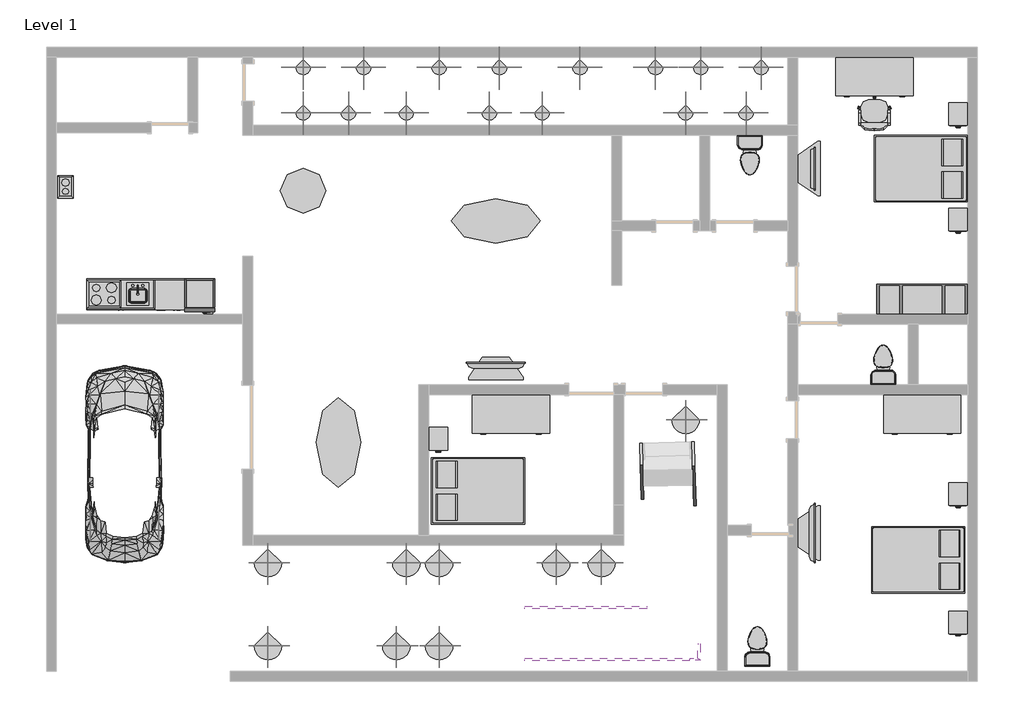
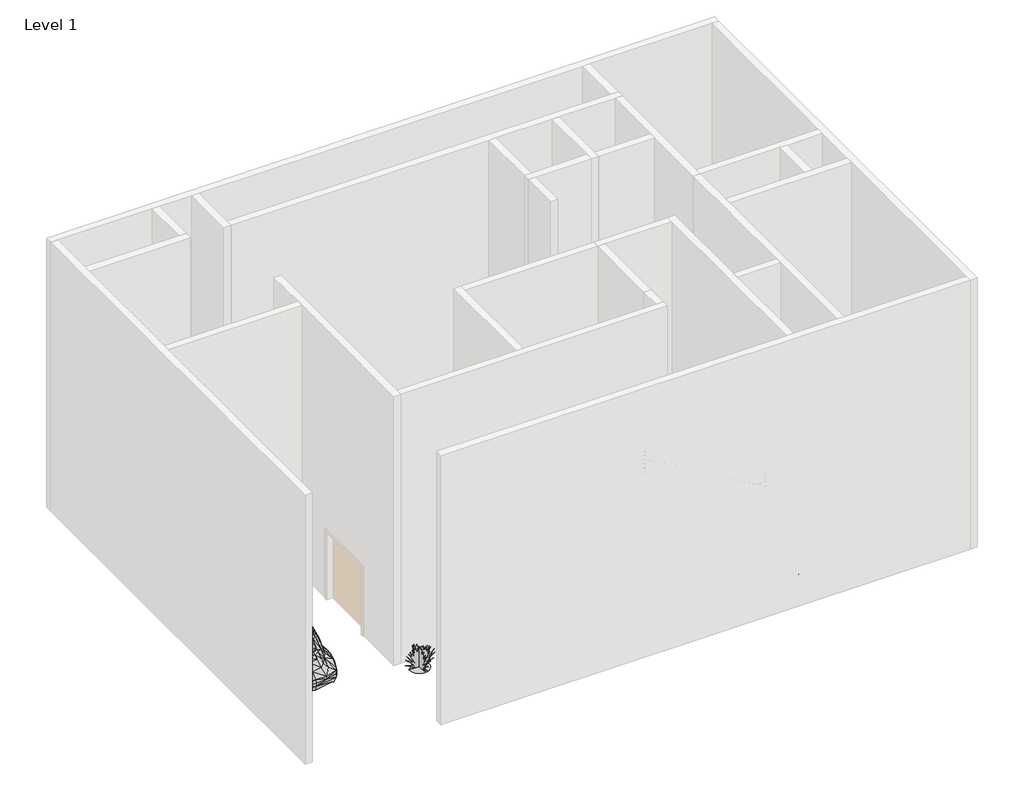
# One storey, part 4 of 4: 24 geographic elements, 23 furniture elements, 6 members, 6 proxies, 4 flow terminals.
"""IFC4 building model written with IfcOpenShell, lengths in millimetres."""

from ifc_helpers import new_model, si_unit, frame, origin, place, context, project, spatial, polyline, outline, extrude, faceted_brep, transform, mapped, element, save
from components import m_cook_top_2_unit_305_x_457mm_ebea1746, m_cook_top_4_unit2_0615_x_500mm_249f3515, m_dishwasher_610_x_610_x_875mm_54ecfc4c, m_kitchenette_medium_1372mm_e05c6bec, m_rpc_beetle_m_rpc_beetle_b6d71803, m_refrigerator_600_x_660mm_a466bf94, m_sink_kitchen_island_450_x_450mm_f969cf2d, m_toilet_domestic_3d_m_toilet_domestic_3d_5cb52bd4, m_toilet_domestic_3d_m_toilet_domestic_3d_183bbd19, m_toilet_domestic_3d_m_toilet_domestic_3d_43425dfb, m_toilet_domestic_3d_m_toilet_domestic_3d_5530cc89, furniture_40ec15d9, furniture_0810mm_56245f3a, furniture_1190mm_d9bcc661, m_bed_box_1346_x_1880mm_double_b32eb57e, m_cabinet_file_2_drawer_0380_x_0457mm_9eec7cff, m_chair_executive_m_chair_executive_8d69e98c, m_counter_top_w_sink_hole_600mm_depth_0a237b63, m_desk_1525_x_762mm_8f660baf, m_entertainment_center_1830_x_1830_x_0610mm_f77a9b93, m_table_dining_round_w_chairs_0915mm_diameter_5defa876, m_table_ellipse_1800_x_900mm_fd46d5a5, m_rpc_plant_tropical_agave_0_45_meters_eb57889b, m_rpc_plant_tropical_dagger_0_6_meters_5dc34e47

model = new_model("IFC4")

# Units and contexts
model_context = context("Model", 3, world=origin())
ifc_project = project(units=[si_unit("LENGTHUNIT", "METRE", prefix="MILLI")], contexts=[model_context])

# Site, building, storey
site = spatial("IfcSite", under=ifc_project)
building = spatial("IfcBuilding", under=site)
storey = spatial("IfcBuildingStorey", under=building, Name="Level 1", Elevation=0.0)

# Proxies
placement = place(None, origin())
m_cook_top_2_unit_305_x_457mm_shape = m_cook_top_2_unit_305_x_457mm_ebea1746(model_context)
element("IfcBuildingElementProxy", 1, Name="M_Cook Top-2 Unit : 305 x 457mm", ObjectType="M_Cook Top-2 Unit : 305 x 457mm", at=placement, inside=storey, context=model_context, shape_type="MappedRepresentation", body=[
    mapped(m_cook_top_2_unit_305_x_457mm_shape, transform((-9406.4268643, 7109.0723156, 0.0), x_axis=(1.0, 0.0, 0.0), y_axis=(0.0, 1.0, 0.0), z_axis=(0.0, 0.0, 1.0))),
])
m_cook_top_4_unit2_0615_x_500mm_shape = m_cook_top_4_unit2_0615_x_500mm_249f3515(model_context)
element("IfcBuildingElementProxy", 2, Name="M_Cook Top-4 Unit2 : 0615 x 500mm", ObjectType="M_Cook Top-4 Unit2 : 0615 x 500mm", at=placement, inside=storey, context=model_context, shape_type="MappedRepresentation", body=[
    mapped(m_cook_top_4_unit2_0615_x_500mm_shape, transform((-8555.8268643, 4978.8971112, 0.0), x_axis=(1.0, 0.0, 0.0), y_axis=(0.0, 1.0, 0.0), z_axis=(0.0, 0.0, 1.0))),
])
m_dishwasher_610_x_610_x_875mm_shape = m_dishwasher_610_x_610_x_875mm_54ecfc4c(model_context)
element("IfcBuildingElementProxy", 3, Name="M_Dishwasher : 610 x 610 x 875mm", ObjectType="M_Dishwasher : 610 x 610 x 875mm", at=placement, inside=storey, context=model_context, shape_type="MappedRepresentation", body=[
    mapped(m_dishwasher_610_x_610_x_875mm_shape, transform((-7606.3443328, 4712.2475464, 0.0), x_axis=(1.0, 0.0, 0.0), y_axis=(0.0, 1.0, 0.0), z_axis=(0.0, 0.0, 1.0))),
])
m_kitchenette_medium_1372mm_shape = m_kitchenette_medium_1372mm_e05c6bec(model_context)
element("IfcBuildingElementProxy", 4, Name="M_Kitchenette - Medium : 1372mm", ObjectType="M_Kitchenette - Medium : 1372mm", at=placement, inside=storey, context=model_context, shape_type="MappedRepresentation", body=[
    mapped(m_kitchenette_medium_1372mm_shape, transform((-8231.5645692, 5283.8971112, 0.0), x_axis=(1.0, 0.0, 0.0), y_axis=(0.0, 1.0, 0.0), z_axis=(0.0, 0.0, 1.0))),
])
m_rpc_beetle_m_rpc_beetle_shape = m_rpc_beetle_m_rpc_beetle_b6d71803(model_context)
element("IfcBuildingElementProxy", 5, Name="M_RPC Beetle : M_RPC Beetle", ObjectType="M_RPC Beetle : M_RPC Beetle", at=placement, inside=storey, context=model_context, shape_type="MappedRepresentation", body=[
    mapped(m_rpc_beetle_m_rpc_beetle_shape, transform((-8136.4268643, 306.6971112, 0.0), x_axis=(1.0, 0.0, 0.0), y_axis=(0.0, 1.0, 0.0), z_axis=(0.0, 0.0, 1.0))),
])
m_refrigerator_600_x_660mm_shape = m_refrigerator_600_x_660mm_a466bf94(model_context)
element("IfcBuildingElementProxy", 6, Name="M_Refrigerator : 600 x 660mm", ObjectType="M_Refrigerator : 600 x 660mm", at=placement, inside=storey, context=model_context, shape_type="MappedRepresentation", body=[
    mapped(m_refrigerator_600_x_660mm_shape, transform((-6565.0257216, 4987.682021, 0.0), x_axis=(1.0, 0.0, 0.0), y_axis=(0.0, 1.0, 0.0), z_axis=(0.0, 0.0, 1.0))),
])

# Flow terminals
m_sink_kitchen_island_450_x_450mm_shape = m_sink_kitchen_island_450_x_450mm_f969cf2d(model_context)
element("IfcFlowTerminal", 7, ObjectType="M_Sink Kitchen-Island : 450 x 450mm", at=placement, inside=storey, context=model_context, shape_type="MappedRepresentation", body=[
    mapped(m_sink_kitchen_island_450_x_450mm_shape, transform((-7885.5161048, 4976.5517101, 0.0), x_axis=(1.0, 0.0, 0.0), y_axis=(0.0, 1.0, 0.0), z_axis=(0.0, 0.0, 1.0))),
])
m_toilet_domestic_3d_m_toilet_domestic_3d_shape = m_toilet_domestic_3d_m_toilet_domestic_3d_5cb52bd4(model_context)
m_toilet_domestic_3d_m_toilet_domestic_3d_2_shape = m_toilet_domestic_3d_m_toilet_domestic_3d_183bbd19(model_context)
element("IfcFlowTerminal", 8, ObjectType="M_Toilet-Domestic-3D : M_Toilet-Domestic-3D", at=placement, inside=storey, context=model_context, shape_type="MappedRepresentation", body=[
    mapped(m_toilet_domestic_3d_m_toilet_domestic_3d_shape, transform((4486.3771084, 7686.0010839, 0.0), x_axis=(1.0, 0.0, 0.0), y_axis=(0.0, 1.0, 0.0), z_axis=(0.0, 0.0, 1.0))),
    mapped(m_toilet_domestic_3d_m_toilet_domestic_3d_2_shape, transform((4486.3771084, 7686.0010839, 0.0), x_axis=(1.0, 0.0, 0.0), y_axis=(0.0, 1.0, 0.0), z_axis=(0.0, 0.0, 1.0))),
])
element("IfcFlowTerminal", 9, ObjectType="M_Toilet-Domestic-3D : M_Toilet-Domestic-3D", at=placement, inside=storey, context=model_context, shape_type="MappedRepresentation", body=[
    mapped(m_toilet_domestic_3d_m_toilet_domestic_3d_shape, transform((4637.5691631, -2043.4068614, 0.0), x_axis=(-1.0000000000000004, 0.0, 0.0), y_axis=(0.0, -1.0000000000000004, 0.0), z_axis=(0.0, 0.0, 1.0))),
    mapped(m_toilet_domestic_3d_m_toilet_domestic_3d_2_shape, transform((4637.5691631, -2043.4068614, 0.0), x_axis=(-1.0000000000000004, 0.0, 0.0), y_axis=(0.0, -1.0000000000000004, 0.0), z_axis=(0.0, 0.0, 1.0))),
])
m_toilet_domestic_3d_m_toilet_domestic_3d_3_shape = m_toilet_domestic_3d_m_toilet_domestic_3d_43425dfb(model_context)
m_toilet_domestic_3d_m_toilet_domestic_3d_4_shape = m_toilet_domestic_3d_m_toilet_domestic_3d_5530cc89(model_context)
element("IfcFlowTerminal", 10, ObjectType="M_Toilet-Domestic-3D : M_Toilet-Domestic-3D", at=placement, inside=storey, context=model_context, shape_type="MappedRepresentation", body=[
    mapped(m_toilet_domestic_3d_m_toilet_domestic_3d_3_shape, transform((7177.1771084, 3642.6010839, 0.0), x_axis=(1.0, 0.0, 0.0), y_axis=(0.0, 1.0, 0.0), z_axis=(0.0, 0.0, 1.0))),
    mapped(m_toilet_domestic_3d_m_toilet_domestic_3d_4_shape, transform((7177.1771084, 3642.6010839, 0.0), x_axis=(1.0, 0.0, 0.0), y_axis=(0.0, 1.0, 0.0), z_axis=(0.0, 0.0, 1.0))),
])

# Furniture
furniture_shape = furniture_40ec15d9(model_context)
element("IfcFurniture", 11, at=placement, inside=storey, context=model_context, shape_type="MappedRepresentation", body=[
    mapped(furniture_shape, transform((5449.3731357, 7382.5091092, 0.0), x_axis=(0.0, 1.0000000000000002, 0.0), y_axis=(-1.0000000000000002, 0.0, 0.0), z_axis=(0.0, 0.0, 1.0))),
])
element("IfcFurniture", 12, at=placement, inside=storey, context=model_context, shape_type="MappedRepresentation", body=[
    mapped(furniture_shape, transform((5449.3731357, 25.9091092, 0.0), x_axis=(0.0, 1.0000000000000009, 0.0), y_axis=(-1.0000000000000009, 0.0, 0.0), z_axis=(0.0, 0.0, 1.0))),
])
element("IfcFurniture", 13, at=placement, inside=storey, context=model_context, shape_type="MappedRepresentation", body=[
    mapped(furniture_shape, transform((-768.6148663, 3703.8971112, 0.0), x_axis=(1.0, 0.0, 0.0), y_axis=(0.0, 1.0, 0.0), z_axis=(0.0, 0.0, 1.0))),
])
furniture_0810mm_shape = furniture_0810mm_56245f3a(model_context)
element("IfcFurniture", 14, ObjectType="0810mm", at=placement, inside=storey, context=model_context, shape_type="MappedRepresentation", body=[
    mapped(furniture_0810mm_shape, transform((5737.9117594, 7511.6416254, 0.0), x_axis=(0.0, 1.0, 0.0), y_axis=(-1.0, 0.0, 0.0), z_axis=(0.0, 0.0, 1.0))),
])
furniture_1190mm_shape = furniture_1190mm_d9bcc661(model_context)
element("IfcFurniture", 15, ObjectType="1190mm", at=placement, inside=storey, context=model_context, shape_type="MappedRepresentation", body=[
    mapped(furniture_1190mm_shape, transform((5737.9117594, 155.0416254, 0.0), x_axis=(0.0, 1.0, 0.0), y_axis=(-1.0, 0.0, 0.0), z_axis=(0.0, 0.0, 1.0))),
])
element("IfcFurniture", 16, ObjectType="1190mm", at=placement, inside=storey, context=model_context, shape_type="MappedRepresentation", body=[
    mapped(furniture_1190mm_shape, transform((-647.3713784, 3532.4357349, 0.0), x_axis=(-1.0000000000000002, 0.0, 0.0), y_axis=(0.0, -1.0000000000000002, 0.0), z_axis=(0.0, 0.0, 1.0))),
])
m_bed_box_1346_x_1880mm_double_shape = m_bed_box_1346_x_1880mm_double_b32eb57e(model_context)
element("IfcFurniture", 17, ObjectType="M_Bed-Box : 1346 x 1880mm - Double", at=placement, inside=storey, context=model_context, shape_type="MappedRepresentation", body=[
    mapped(m_bed_box_1346_x_1880mm_double_shape, transform((8174.4026439, 7846.8495702, 0.0), x_axis=(0.0, -1.0000000000000007, 0.0), y_axis=(1.0000000000000007, 0.0, 0.0), z_axis=(0.0, 0.0, 1.0))),
])
element("IfcFurniture", 18, ObjectType="M_Bed-Box : 1346 x 1880mm - Double", at=placement, inside=storey, context=model_context, shape_type="MappedRepresentation", body=[
    mapped(m_bed_box_1346_x_1880mm_double_shape, transform((8119.0026439, -51.1504298, 0.0), x_axis=(0.0, -1.0000000000000004, 0.0), y_axis=(1.0000000000000004, 0.0, 0.0), z_axis=(0.0, 0.0, 1.0))),
])
element("IfcFurniture", 19, ObjectType="M_Bed-Box : 1346 x 1880mm - Double", at=placement, inside=storey, context=model_context, shape_type="MappedRepresentation", body=[
    mapped(m_bed_box_1346_x_1880mm_double_shape, transform((-1238.0563725, 662.9446522, 0.0), x_axis=(0.0, 0.9999999999999999, 0.0), y_axis=(-0.9999999999999999, 0.0, 0.0), z_axis=(0.0, 0.0, 1.0))),
])
m_cabinet_file_2_drawer_0380_x_0457mm_shape = m_cabinet_file_2_drawer_0380_x_0457mm_9eec7cff(model_context)
element("IfcFurniture", 20, ObjectType="M_Cabinet-File 2 Drawer : 0380 x 0457mm", at=placement, inside=storey, context=model_context, shape_type="MappedRepresentation", body=[
    mapped(m_cabinet_file_2_drawer_0380_x_0457mm_shape, transform((8817.8695828, 6622.5314113, 0.0), x_axis=(1.0, 0.0, 0.0), y_axis=(0.0, 1.0, 0.0), z_axis=(0.0, 0.0, 1.0))),
])
element("IfcFurniture", 21, ObjectType="M_Cabinet-File 2 Drawer : 0380 x 0457mm", at=placement, inside=storey, context=model_context, shape_type="MappedRepresentation", body=[
    mapped(m_cabinet_file_2_drawer_0380_x_0457mm_shape, transform((8817.8695828, 8751.3314113, 0.0), x_axis=(1.0, 0.0, 0.0), y_axis=(0.0, 1.0, 0.0), z_axis=(0.0, 0.0, 1.0))),
])
element("IfcFurniture", 22, ObjectType="M_Cabinet-File 2 Drawer : 0380 x 0457mm", at=placement, inside=storey, context=model_context, shape_type="MappedRepresentation", body=[
    mapped(m_cabinet_file_2_drawer_0380_x_0457mm_shape, transform((8817.8695828, 1080.7314113, 0.0), x_axis=(1.0, 0.0, 0.0), y_axis=(0.0, 1.0, 0.0), z_axis=(0.0, 0.0, 1.0))),
])
element("IfcFurniture", 23, ObjectType="M_Cabinet-File 2 Drawer : 0380 x 0457mm", at=placement, inside=storey, context=model_context, shape_type="MappedRepresentation", body=[
    mapped(m_cabinet_file_2_drawer_0380_x_0457mm_shape, transform((8817.8695828, -1510.0685887, 0.0), x_axis=(1.0, 0.0, 0.0), y_axis=(0.0, 1.0, 0.0), z_axis=(0.0, 0.0, 1.0))),
])
element("IfcFurniture", 24, ObjectType="M_Cabinet-File 2 Drawer : 0380 x 0457mm", at=placement, inside=storey, context=model_context, shape_type="MappedRepresentation", body=[
    mapped(m_cabinet_file_2_drawer_0380_x_0457mm_shape, transform((-1676.5304172, 2198.3314113, 0.0), x_axis=(1.0, 0.0, 0.0), y_axis=(0.0, 1.0, 0.0), z_axis=(0.0, 0.0, 1.0))),
])
m_chair_executive_m_chair_executive_shape = m_chair_executive_m_chair_executive_8d69e98c(model_context)
element("IfcFurniture", 25, ObjectType="M_Chair-Executive : M_Chair-Executive", at=placement, inside=storey, context=model_context, shape_type="MappedRepresentation", body=[
    mapped(m_chair_executive_m_chair_executive_shape, transform((6857.2823161, 8620.5512096, 0.0), x_axis=(1.0, 0.0, 0.0), y_axis=(0.0, 1.0, 0.0), z_axis=(0.0, 0.0, 1.0))),
])
m_counter_top_w_sink_hole_600mm_depth_shape = m_counter_top_w_sink_hole_600mm_depth_0a237b63(model_context)
element("IfcFurniture", 26, ObjectType="M_Counter Top w Sink Hole : 600mm Depth", at=placement, inside=storey, context=model_context, shape_type="MappedRepresentation", body=[
    mapped(m_counter_top_w_sink_hole_600mm_depth_shape, transform((-7698.3645692, 5283.8971112, 0.0), x_axis=(1.0, 0.0, 0.0), y_axis=(0.0, 1.0, 0.0), z_axis=(0.0, 0.0, 1.0))),
])
m_desk_1525_x_762mm_shape = m_desk_1525_x_762mm_8f660baf(model_context)
element("IfcFurniture", 27, ObjectType="M_Desk : 1525 x 762mm", at=placement, inside=storey, context=model_context, shape_type="MappedRepresentation", body=[
    mapped(m_desk_1525_x_762mm_shape, transform((6236.2731357, 8996.6971112, 0.0), x_axis=(1.0, 0.0, 0.0), y_axis=(0.0, 1.0, 0.0), z_axis=(0.0, 0.0, 1.0))),
])
element("IfcFurniture", 28, ObjectType="M_Desk : 1525 x 762mm", at=placement, inside=storey, context=model_context, shape_type="MappedRepresentation", body=[
    mapped(m_desk_1525_x_762mm_shape, transform((7202.9731357, 2184.6971112, 0.0), x_axis=(1.0, 0.0, 0.0), y_axis=(0.0, 1.0, 0.0), z_axis=(0.0, 0.0, 1.0))),
])
element("IfcFurniture", 29, ObjectType="M_Desk : 1525 x 762mm", at=placement, inside=storey, context=model_context, shape_type="MappedRepresentation", body=[
    mapped(m_desk_1525_x_762mm_shape, transform((-1101.1268643, 2184.6971112, 0.0), x_axis=(1.0, 0.0, 0.0), y_axis=(0.0, 1.0, 0.0), z_axis=(0.0, 0.0, 1.0))),
])
m_entertainment_center_1830_x_1830_x_0610mm_shape = m_entertainment_center_1830_x_1830_x_0610mm_f77a9b93(model_context)
element("IfcFurniture", 30, ObjectType="M_Entertainment center : 1830 x 1830 x 0610mm", at=placement, inside=storey, context=model_context, shape_type="MappedRepresentation", body=[
    mapped(m_entertainment_center_1830_x_1830_x_0610mm_shape, transform((7964.9731357, 5277.2971112, 0.0), x_axis=(1.0, 0.0, 0.0), y_axis=(0.0, 1.0, 0.0), z_axis=(0.0, 0.0, 1.0))),
])
m_table_dining_round_w_chairs_0915mm_diameter_shape = m_table_dining_round_w_chairs_0915mm_diameter_5defa876(model_context)
element("IfcFurniture", 31, ObjectType="M_Table-Dining Round w Chairs : 0915mm Diameter", at=placement, inside=storey, context=model_context, shape_type="MappedRepresentation", body=[
    mapped(m_table_dining_round_w_chairs_0915mm_diameter_shape, transform((-4636.5088315, 7246.3757997, 0.0), x_axis=(1.0, 0.0, 0.0), y_axis=(0.0, 1.0, 0.0), z_axis=(0.0, 0.0, 1.0))),
])
m_table_ellipse_1800_x_900mm_shape = m_table_ellipse_1800_x_900mm_fd46d5a5(model_context)
element("IfcFurniture", 32, ObjectType="M_Table-Ellipse : 1800 x 900mm", at=placement, inside=storey, context=model_context, shape_type="MappedRepresentation", body=[
    mapped(m_table_ellipse_1800_x_900mm_shape, transform((-643.4268643, 6451.8971112, 0.0), x_axis=(1.0, 0.0, 0.0), y_axis=(0.0, 1.0, 0.0), z_axis=(0.0, 0.0, 1.0))),
])
element("IfcFurniture", 33, ObjectType="M_Table-Ellipse : 1800 x 900mm", at=placement, inside=storey, context=model_context, shape_type="MappedRepresentation", body=[
    mapped(m_table_ellipse_1800_x_900mm_shape, transform((-3821.6268643, 1979.8971112, 0.0), x_axis=(0.0, 1.0000000000000002, 0.0), y_axis=(-1.0000000000000002, 0.0, 0.0), z_axis=(0.0, 0.0, 1.0))),
])

# Geographic elements
m_rpc_plant_tropical_agave_0_45_meters_shape = m_rpc_plant_tropical_agave_0_45_meters_eb57889b(model_context)
element("IfcGeographicElement", 34, ObjectType="M_RPC Plant - Tropical : Agave - 0.45 Meters", at=placement, inside=storey, context=model_context, shape_type="MappedRepresentation", body=[
    mapped(m_rpc_plant_tropical_agave_0_45_meters_shape, transform((-4531.4235354, 9553.8971112, 0.0), x_axis=(1.0, 0.0, 0.0), y_axis=(0.0, 1.0, 0.0), z_axis=(0.0, 0.0, 1.0))),
])
element("IfcGeographicElement", 35, ObjectType="M_RPC Plant - Tropical : Agave - 0.45 Meters", at=placement, inside=storey, context=model_context, shape_type="MappedRepresentation", body=[
    mapped(m_rpc_plant_tropical_agave_0_45_meters_shape, transform((-3312.2235354, 9553.8971112, 0.0), x_axis=(1.0, 0.0, 0.0), y_axis=(0.0, 1.0, 0.0), z_axis=(0.0, 0.0, 1.0))),
])
element("IfcGeographicElement", 36, ObjectType="M_RPC Plant - Tropical : Agave - 0.45 Meters", at=placement, inside=storey, context=model_context, shape_type="MappedRepresentation", body=[
    mapped(m_rpc_plant_tropical_agave_0_45_meters_shape, transform((-1788.2235354, 9553.8971112, 0.0), x_axis=(1.0, 0.0, 0.0), y_axis=(0.0, 1.0, 0.0), z_axis=(0.0, 0.0, 1.0))),
])
element("IfcGeographicElement", 37, ObjectType="M_RPC Plant - Tropical : Agave - 0.45 Meters", at=placement, inside=storey, context=model_context, shape_type="MappedRepresentation", body=[
    mapped(m_rpc_plant_tropical_agave_0_45_meters_shape, transform((-569.0235354, 9553.8971112, 0.0), x_axis=(1.0, 0.0, 0.0), y_axis=(0.0, 1.0, 0.0), z_axis=(0.0, 0.0, 1.0))),
])
element("IfcGeographicElement", 38, ObjectType="M_RPC Plant - Tropical : Agave - 0.45 Meters", at=placement, inside=storey, context=model_context, shape_type="MappedRepresentation", body=[
    mapped(m_rpc_plant_tropical_agave_0_45_meters_shape, transform((1054.9764646, 9553.8971112, 0.0), x_axis=(1.0, 0.0, 0.0), y_axis=(0.0, 1.0, 0.0), z_axis=(0.0, 0.0, 1.0))),
])
element("IfcGeographicElement", 39, ObjectType="M_RPC Plant - Tropical : Agave - 0.45 Meters", at=placement, inside=storey, context=model_context, shape_type="MappedRepresentation", body=[
    mapped(m_rpc_plant_tropical_agave_0_45_meters_shape, transform((2578.9764646, 9553.8971112, 0.0), x_axis=(1.0, 0.0, 0.0), y_axis=(0.0, 1.0, 0.0), z_axis=(0.0, 0.0, 1.0))),
])
element("IfcGeographicElement", 40, ObjectType="M_RPC Plant - Tropical : Agave - 0.45 Meters", at=placement, inside=storey, context=model_context, shape_type="MappedRepresentation", body=[
    mapped(m_rpc_plant_tropical_agave_0_45_meters_shape, transform((4712.5764646, 9553.8971112, 0.0), x_axis=(1.0, 0.0, 0.0), y_axis=(0.0, 1.0, 0.0), z_axis=(0.0, 0.0, 1.0))),
])
element("IfcGeographicElement", 41, ObjectType="M_RPC Plant - Tropical : Agave - 0.45 Meters", at=placement, inside=storey, context=model_context, shape_type="MappedRepresentation", body=[
    mapped(m_rpc_plant_tropical_agave_0_45_meters_shape, transform((-4531.4235354, 8639.4971112, 0.0), x_axis=(1.0, 0.0, 0.0), y_axis=(0.0, 1.0, 0.0), z_axis=(0.0, 0.0, 1.0))),
])
element("IfcGeographicElement", 42, ObjectType="M_RPC Plant - Tropical : Agave - 0.45 Meters", at=placement, inside=storey, context=model_context, shape_type="MappedRepresentation", body=[
    mapped(m_rpc_plant_tropical_agave_0_45_meters_shape, transform((-2450.2235354, 8639.4971112, 0.0), x_axis=(1.0, 0.0, 0.0), y_axis=(0.0, 1.0, 0.0), z_axis=(0.0, 0.0, 1.0))),
])
element("IfcGeographicElement", 43, ObjectType="M_RPC Plant - Tropical : Agave - 0.45 Meters", at=placement, inside=storey, context=model_context, shape_type="MappedRepresentation", body=[
    mapped(m_rpc_plant_tropical_agave_0_45_meters_shape, transform((-773.8235354, 8639.4971112, 0.0), x_axis=(1.0, 0.0, 0.0), y_axis=(0.0, 1.0, 0.0), z_axis=(0.0, 0.0, 1.0))),
])
element("IfcGeographicElement", 44, ObjectType="M_RPC Plant - Tropical : Agave - 0.45 Meters", at=placement, inside=storey, context=model_context, shape_type="MappedRepresentation", body=[
    mapped(m_rpc_plant_tropical_agave_0_45_meters_shape, transform((-3617.0235354, 8639.4971112, 0.0), x_axis=(1.0, 0.0, 0.0), y_axis=(0.0, 1.0, 0.0), z_axis=(0.0, 0.0, 1.0))),
])
element("IfcGeographicElement", 45, ObjectType="M_RPC Plant - Tropical : Agave - 0.45 Meters", at=placement, inside=storey, context=model_context, shape_type="MappedRepresentation", body=[
    mapped(m_rpc_plant_tropical_agave_0_45_meters_shape, transform((3188.5764646, 8639.4971112, 0.0), x_axis=(1.0, 0.0, 0.0), y_axis=(0.0, 1.0, 0.0), z_axis=(0.0, 0.0, 1.0))),
])
element("IfcGeographicElement", 46, ObjectType="M_RPC Plant - Tropical : Agave - 0.45 Meters", at=placement, inside=storey, context=model_context, shape_type="MappedRepresentation", body=[
    mapped(m_rpc_plant_tropical_agave_0_45_meters_shape, transform((4407.7764646, 8639.4971112, 0.0), x_axis=(1.0, 0.0, 0.0), y_axis=(0.0, 1.0, 0.0), z_axis=(0.0, 0.0, 1.0))),
])
element("IfcGeographicElement", 47, ObjectType="M_RPC Plant - Tropical : Agave - 0.45 Meters", at=placement, inside=storey, context=model_context, shape_type="MappedRepresentation", body=[
    mapped(m_rpc_plant_tropical_agave_0_45_meters_shape, transform((3493.3764646, 9553.8971112, 0.0), x_axis=(1.0, 0.0, 0.0), y_axis=(0.0, 1.0, 0.0), z_axis=(0.0, 0.0, 1.0))),
])
element("IfcGeographicElement", 48, ObjectType="M_RPC Plant - Tropical : Agave - 0.45 Meters", at=placement, inside=storey, context=model_context, shape_type="MappedRepresentation", body=[
    mapped(m_rpc_plant_tropical_agave_0_45_meters_shape, transform((292.9764646, 8639.4971112, 0.0), x_axis=(1.0, 0.0, 0.0), y_axis=(0.0, 1.0, 0.0), z_axis=(0.0, 0.0, 1.0))),
])
m_rpc_plant_tropical_dagger_0_6_meters_shape = m_rpc_plant_tropical_dagger_0_6_meters_5dc34e47(model_context)
element("IfcGeographicElement", 49, ObjectType="M_RPC Plant - Tropical : Dagger - 0.6 Meters", at=placement, inside=storey, context=model_context, shape_type="MappedRepresentation", body=[
    mapped(m_rpc_plant_tropical_dagger_0_6_meters_shape, transform((-1788.2235354, -450.5028888, 0.0), x_axis=(1.0, 0.0, 0.0), y_axis=(0.0, 1.0, 0.0), z_axis=(0.0, 0.0, 1.0))),
])
element("IfcGeographicElement", 50, ObjectType="M_RPC Plant - Tropical : Dagger - 0.6 Meters", at=placement, inside=storey, context=model_context, shape_type="MappedRepresentation", body=[
    mapped(m_rpc_plant_tropical_dagger_0_6_meters_shape, transform((575.5764646, -450.5028888, 0.0), x_axis=(1.0, 0.0, 0.0), y_axis=(0.0, 1.0, 0.0), z_axis=(0.0, 0.0, 1.0))),
])
element("IfcGeographicElement", 51, ObjectType="M_RPC Plant - Tropical : Dagger - 0.6 Meters", at=placement, inside=storey, context=model_context, shape_type="MappedRepresentation", body=[
    mapped(m_rpc_plant_tropical_dagger_0_6_meters_shape, transform((-1788.2235354, -2126.9028888, 0.0), x_axis=(1.0, 0.0, 0.0), y_axis=(0.0, 1.0, 0.0), z_axis=(0.0, 0.0, 1.0))),
])
element("IfcGeographicElement", 52, ObjectType="M_RPC Plant - Tropical : Dagger - 0.6 Meters", at=placement, inside=storey, context=model_context, shape_type="MappedRepresentation", body=[
    mapped(m_rpc_plant_tropical_dagger_0_6_meters_shape, transform((1489.9764646, -450.5028888, 0.0), x_axis=(1.0, 0.0, 0.0), y_axis=(0.0, 1.0, 0.0), z_axis=(0.0, 0.0, 1.0))),
])
element("IfcGeographicElement", 53, ObjectType="M_RPC Plant - Tropical : Dagger - 0.6 Meters", at=placement, inside=storey, context=model_context, shape_type="MappedRepresentation", body=[
    mapped(m_rpc_plant_tropical_dagger_0_6_meters_shape, transform((3188.5764646, 2437.0971112, 0.0), x_axis=(1.0, 0.0, 0.0), y_axis=(0.0, 1.0, 0.0), z_axis=(0.0, 0.0, 1.0))),
])
element("IfcGeographicElement", 54, ObjectType="M_RPC Plant - Tropical : Dagger - 0.6 Meters", at=placement, inside=storey, context=model_context, shape_type="MappedRepresentation", body=[
    mapped(m_rpc_plant_tropical_dagger_0_6_meters_shape, transform((-2450.2235354, -450.5028888, 0.0), x_axis=(1.0, 0.0, 0.0), y_axis=(0.0, 1.0, 0.0), z_axis=(0.0, 0.0, 1.0))),
])
element("IfcGeographicElement", 55, ObjectType="M_RPC Plant - Tropical : Dagger - 0.6 Meters", at=placement, inside=storey, context=model_context, shape_type="MappedRepresentation", body=[
    mapped(m_rpc_plant_tropical_dagger_0_6_meters_shape, transform((-5242.6235354, -450.5028888, 0.0), x_axis=(1.0, 0.0, 0.0), y_axis=(0.0, 1.0, 0.0), z_axis=(0.0, 0.0, 1.0))),
])
element("IfcGeographicElement", 56, ObjectType="M_RPC Plant - Tropical : Dagger - 0.6 Meters", at=placement, inside=storey, context=model_context, shape_type="MappedRepresentation", body=[
    mapped(m_rpc_plant_tropical_dagger_0_6_meters_shape, transform((-5242.6235354, -2126.9028888, 0.0), x_axis=(1.0, 0.0, 0.0), y_axis=(0.0, 1.0, 0.0), z_axis=(0.0, 0.0, 1.0))),
])
element("IfcGeographicElement", 57, ObjectType="M_RPC Plant - Tropical : Dagger - 0.6 Meters", at=placement, inside=storey, context=model_context, shape_type="MappedRepresentation", body=[
    mapped(m_rpc_plant_tropical_dagger_0_6_meters_shape, transform((-2651.8235354, -2126.9028888, 0.0), x_axis=(1.0, 0.0, 0.0), y_axis=(0.0, 1.0, 0.0), z_axis=(0.0, 0.0, 1.0))),
])

# Members
element("IfcMember", 58, ObjectType="Stringer - 50mm Width", at=placement, inside=storey, context=model_context, shape_type="SweptSolid", body=[
    extrude(outline(polyline([(228.5743526, -400.0), (0.0, 0.0), (4698.3521163, 0.0), (4926.9264689, -400.0), (228.5743526, -400.0)])), frame((3312.7261016, 1995.8360342, 461.7441657), z_axis=(0.9995887272032868, 0.02867710669005952, 0.0), x_axis=(0.02489862281365917, -0.8678833243678472, 0.496143722993849)), (0.0, 0.0, 1.0), 50.0),
])
element("IfcMember", 59, ObjectType="Stringer - 50mm Width", at=placement, inside=storey, context=model_context, shape_type="SweptSolid", body=[
    extrude(outline(polyline([(3429.7085988, -2081.7854195), (3479.6880351, -2080.3515642), (3489.4678507, -2421.2434646), (3438.01674, -2371.3796371), (3429.7085988, -2081.7854195)])), frame((0.0, 0.0, 2792.8020766), z_axis=(0.0, 0.0, 1.0), x_axis=(1.0, 0.0, 0.0)), (0.0, 0.0, 1.0), 460.7018935),
])
element("IfcMember", 60, ObjectType="Stringer - 50mm Width", at=placement, inside=storey, context=model_context, shape_type="SweptSolid", body=[
    extrude(outline(polyline([(3438.01674, -2371.3796371), (3489.4678507, -2421.2434646), (3267.2772333, -2421.832281), (3267.1447312, -2371.8324566), (3438.01674, -2371.3796371)])), frame((0.0, 0.0, 2792.8020766), z_axis=(0.0, 0.0, 1.0), x_axis=(1.0, 0.0, 0.0)), (0.0, 0.0, 1.0), 460.7018935),
])
element("IfcMember", 61, ObjectType="Stringer - 50mm Width", at=placement, inside=storey, context=model_context, shape_type="Brep", body=[
    faceted_brep([(2263.1321674, 1965.7243329, 899.4881711), (2313.1116037, 1967.1581882, 899.4881711), (2313.1116037, 1967.1581882, 412.6027883), (2263.1321674, 1965.7243329, 412.6027883), (2357.5168849, -1324.2135481, 3183.5794989), (2407.5336543, -1324.0810011, 3184.4829528), (2407.5336543, -1324.0810011, 2697.5975699), (2357.5168849, -1324.2135481, 2696.6941161)], [[[0, 1, 2, 3]], [[1, 0, 4, 5]], [[2, 1, 5, 6]], [[3, 2, 6, 7]], [[0, 3, 7, 4]], [[4, 7, 6, 5]]]),
])
element("IfcMember", 62, ObjectType="Stringer - 50mm Width", at=placement, inside=storey, context=model_context, shape_type="Brep", body=[
    faceted_brep([(-60.4595447, -1330.621308, 5119.5436601), (-60.4595447, -1330.621308, 4625.0488257), (-60.3270426, -1380.6211324, 4625.0488257), (-60.3270426, -1380.6211324, 5119.5436601), (2408.9679956, -1374.0773756, 3324.7791638), (2407.5336543, -1324.0810011, 3325.7253831), (2408.9679956, -1374.0773756, 2830.2843294), (2407.5336543, -1324.0810011, 2831.2305488)], [[[0, 1, 2, 3]], [[4, 5, 0, 3]], [[6, 4, 3, 2]], [[7, 6, 2, 1]], [[5, 7, 1, 0]], [[5, 4, 6, 7]]]),
])
element("IfcMember", 63, ObjectType="Stringer - 50mm Width", at=placement, inside=storey, context=model_context, shape_type="SweptSolid", body=[
    extrude(outline(polyline([(-219.4431203, -405.0814136), (0.0, 0.0), (3781.3559532, -1e-07), (3561.912833, -405.0814136), (-219.4431203, -405.0814136)])), frame((3267.2772333, -2421.832281, 3253.5039701), z_axis=(-0.002650041281452813, 0.9999964886344386, 0.0), x_axis=(-0.8792670421400772, -0.002330102140932527, 0.4763234607178745)), (0.0, 0.0, 1.0), 50.0),
])

save(model, "model.ifc")

# Revit data of these elements
# Type "M_Cook Top-2 Unit : 305 x 457mm"
#   Counter Height = 900 mm
#   Depth = 457 mm
#   Width = 305 mm
#   Burner Material = Steel, Chrome Plated
#   Cooktop Material = Steel, Polished
#   Default Elevation = 0
# Type "M_Cook Top-4 Unit2 : 0615 x 500mm"
#   Depth = 500 mm
#   Width = 615 mm
#   Burner Material = Steel, Chrome Plated
#   Cooktop Material = Steel, Polished
#   Default Elevation = 0
#   Assembly Code = ""
# Type "M_Dishwasher : 610 x 610 x 875mm"
#   Label = "DW"
#   Depth = 610 mm
#   Height = 875 mm
#   Width = 610 mm
#   Dishwasher Material = Steel, Paint Finish, Ivory, Glossy
#   Panel Face Material = Plastic, Opaque Black
#   Default Elevation = 0
# Type "M_Kitchenette - Medium : 1372mm"
#   Counter Length = 1980 mm
#   Cabinet Width = 1372 mm
#   Cabinet Height = 900 mm
#   Cabinet Depth = 610 mm
#   Toe Depth = 35 mm
#   Toe Height = 100 mm
#   Cabinet Material = Cabinets
#   Door/Drawer Material = Cabinets
#   Handle Material = Cabinets - Handles
#   Default Elevation = 0
# Type "M_RPC Beetle : M_RPC Beetle"
#   built-in parameter 1005198 = "{2, 15},{39, RPC-16-0U6E-L4EG-ENH1-J3KF-SVEL-0TX4-C0},{1, 0},{1, 0},{2, 18},{1, 8},{5, Color},{1, 0},{1, 0},{3, 0.8},{3, 0.8},{3, 0.8},{1, 8},{7, BBoxMin},{1, 0},{1, 0},{1, 0},{1, 0},{1, 0},{1, 8},{7, BBoxMax},{1, 0},{1, 0},{1, 0},{1, 0},{1, 0},{2, 11},{9, RPCTypeId},{1, 0},{1, 0},{39, RPC-16-0U6E-L4EG-ENH1-J3KF-SVEL-0TX4-C0},{1, 6},{14, RPCPlantHeight},{1, 0},{1, 0},{4, 4.92},{2, 11},{7, keyword},{1, 0},{1, 0},{39, :RPCs:Auto_Economy/Midsize:Geometry:RPC},{2, 11},{8, category},{1, 0},{1, 0},{20, Auto_Economy/Midsize},{2, 11},{12, LocalizedUID},{1, 0},{1, 0},{13, VW Beetle [4]},{2, 14},{6, Height},{1, 0},{1, 0},{4, 4.92},{1, 2},{16, Cast Reflections},{1, 0},{1, 0},{1, 0},{1, 4},{12, Transparency},{1, 0},{1, 0},{2, 18},{1, 4},{7, Tinting},{1, 0},{1, 0},{2, 50},{1, 2},{11, Use Tinting},{1, 0},{1, 0},{1, 0},{1, 2},{13, License Plate},{1, 0},{1, 0},{1, 0},{2, 11},{21, License Plate Texture},{1, 0},{1, 0},{64, __RPC:/object data/textures/car/plate/textures/default/rgb/0/0/0},{2, 11},{23, i_License Plate Texture},{1, 0},{1, 0},{0, },{1, 2},{12, Custom Plate},{1, 0},{1, 0},{1, 0},{2, 11},{23, License Plate File Name},{1, 0},{1, 0},{0, },{21, assetlibrary_base.fbx},{1, 5},"
#   built-in parameter 1005195 = "RPC-16-0U6E-L4EG-ENH1-J3KF-SVEL-0TX4-C0"
#   Height = 0
# Type "M_Refrigerator : 600 x 660mm"
#   Label = "REF."
#   Depth = 660 mm
#   Height = 1830 mm
#   Width = 600 mm
#   Material = Steel, Paint Finish, Ivory, Matte
#   Description = (empty or 0)
#   Default Elevation = 0
# Type "M_Sink Kitchen-Island : 450 x 450mm"
#   Counter Height [instance default] = 900 mm
#   Depth = 450 mm
#   Width = 450 mm
#   Fixture Material = Steel, Polished
#   Sink Material = Steel, Polished
#   Default Elevation = 0
# Type "M_Toilet-Domestic-3D : M_Toilet-Domestic-3D"
#   Bowl/Basin Material = Porcelain, Linen
#   Seat Material = Laminate, Linen, Matte
#   Default Elevation = 0
# Type
#   Depth = 460 mm
#   Width = 1100 mm
#   Height = 500 mm
#   Finish = Melamine - Gray
#   Default Elevation = 0
# Type "0810mm"
#   SinAng = 0.49 mm
#   L = 705.961 mm
#   H = 397.139 mm
#   Thickness = 110 mm
#   Diagonal = 810 mm
#   CosAng = 0.872 mm
#   Stand [instance default] = yes
#   Default Elevation = 0
# Type "1190mm"
#   SinAng = 0.49 mm
#   L = 1037.152 mm
#   H = 583.452 mm
#   Thickness = 110 mm
#   Diagonal = 1190 mm
#   CosAng = 0.872 mm
#   Stand [instance default] = yes
#   Default Elevation = 0
# Type "M_Bed-Box : 1346 x 1880mm - Double"
#   Length = 1880 mm
#   Width = 1346 mm
#   Frame Material = Birch
#   Mattress Material = Linen, White
#   Default Elevation = 0
# Type "M_Cabinet-File 2 Drawer : 0380 x 0457mm"
#   Depth = 457 mm
#   Height = 734 mm
#   Width = 380 mm
#   Cabinet Material = Steel, Paint Finish, Ivory, Glossy
#   Handle Material = Steel, Chrome Plated
#   Default Elevation = 0
# Type "M_Chair-Executive : M_Chair-Executive"
#   Base/Armd Material = Plastic, Opaque Black
#   Caster Material = Plastic, Opaque Black
#   Seat/Back Material = Textile - Slate Blue
#   Default Elevation = 0
# Type "M_Counter Top w Sink Hole : 600mm Depth"
#   Counter Thickness = 40 mm
#   Depth = 625 mm
#   Height = 900 mm
#   Length [instance default] = 2500 mm
#   Sink Location [instance default] = 1200 mm
#   Sink Location To Wall [instance default] = 100 mm
#   Sink Opening Depth [instance default] = 378 mm
#   Sink Opening Width [instance default] = 587 mm
#   Counter Top Material = none
#   Default Elevation = 0
# Type "M_Desk : 1525 x 762mm"
#   Depth = 762 mm
#   Height = 762 mm
#   Leg Height = 152 mm
#   Width = 1525 mm
#   Body Material = Laminate, Ivory, Matte
#   Handle/Leg Material = Steel, Chrome Plated
#   Top Material = Cherry
#   Default Elevation = 0
#   Assembly Code = ""
# Type "M_Entertainment center : 1830 x 1830 x 0610mm"
#   Center Width = 813 mm
#   Depth = 610 mm
#   Height = 1830 mm
#   Width = 1830 mm
#   Material = Laminate, Ivory, Matte
#   Default Elevation = 0
# Type "M_Table-Dining Round w Chairs : 0915mm Diameter"
#   Radius = 457.5 mm
#   Diameter = 915 mm
#   Height = 762 mm
#   Chairs = 4
#   Base Material = Pine
#   Top Material = Laminate, Linen, Matte
#   Default Elevation = 0
# Type "M_Table-Ellipse : 1800 x 900mm"
#   Half Width = 450 mm
#   Half Length = 900 mm
#   Height = 760 mm
#   Length = 1800 mm
#   Width = 900 mm
#   Base Material = Birch
#   Top Material = Laminate - Black
#   Default Elevation = 0
#   Assembly Code = ""
# Type "M_RPC Plant - Tropical : Agave - 0.45 Meters"
#   built-in parameter 1005198 = "{2, 15},{39, RPC-16-G1GJ-63FX-7K5P-N000-ST1L-LVER-AU},{1, 0},{1, 0},{2, 13},{1, 8},{5, Color},{1, 0},{1, 0},{3, 0.8},{3, 0.8},{3, 0.8},{1, 8},{7, BBoxMin},{1, 0},{1, 0},{1, 0},{1, 0},{1, 0},{1, 8},{7, BBoxMax},{1, 0},{1, 0},{1, 0},{1, 0},{1, 0},{2, 11},{9, RPCTypeId},{1, 0},{1, 0},{39, RPC-16-G1GJ-63FX-7K5P-N000-ST1L-LVER-AU},{1, 6},{14, RPCPlantHeight},{1, 0},{1, 0},{7, 1.47638},{2, 11},{7, keyword},{1, 0},{1, 0},{35, :RPCs:Plants [General]:Geometry:RPC},{2, 11},{8, category},{1, 0},{1, 0},{16, Plants [General]},{2, 11},{12, LocalizedUID},{1, 0},{1, 0},{5, Agave},{2, 14},{6, Height},{1, 0},{1, 0},{7, 1.47638},{1, 2},{16, Cast Reflections},{1, 0},{1, 0},{1, 0},{1, 2},{12, Cast Shadows},{1, 0},{1, 0},{1, 1},{1, 2},{9, Lock View},{1, 0},{1, 0},{1, 0},{1, 4},{5, ViewC},{1, 0},{1, 0},{1, 0},{21, assetlibrary_base.fbx},{1, 5},"
#   built-in parameter 1005195 = "RPC-16-G1GJ-63FX-7K5P-N000-ST1L-LVER-AU"
#   Type Comments = "Agave"
#   Height = 450 mm
#   Description = (empty or 0)
#   Default Elevation = 0
# Type "M_RPC Plant - Tropical : Dagger - 0.6 Meters"
#   built-in parameter 1005198 = "{2, 15},{39, RPC-16-G3A7-NEG0-UH6H-J000-ST1L-LVER-AU},{1, 0},{1, 0},{2, 13},{1, 8},{5, Color},{1, 0},{1, 0},{3, 0.8},{3, 0.8},{3, 0.8},{1, 8},{7, BBoxMin},{1, 0},{1, 0},{1, 0},{1, 0},{1, 0},{1, 8},{7, BBoxMax},{1, 0},{1, 0},{1, 0},{1, 0},{1, 0},{2, 11},{9, RPCTypeId},{1, 0},{1, 0},{39, RPC-16-G3A7-NEG0-UH6H-J000-ST1L-LVER-AU},{1, 6},{14, RPCPlantHeight},{1, 0},{1, 0},{6, 1.9685},{2, 11},{7, keyword},{1, 0},{1, 0},{35, :RPCs:Plants [General]:Geometry:RPC},{2, 11},{8, category},{1, 0},{1, 0},{16, Plants [General]},{2, 11},{12, LocalizedUID},{1, 0},{1, 0},{6, Dagger},{2, 14},{6, Height},{1, 0},{1, 0},{6, 1.9685},{1, 2},{16, Cast Reflections},{1, 0},{1, 0},{1, 0},{1, 2},{12, Cast Shadows},{1, 0},{1, 0},{1, 1},{1, 2},{9, Lock View},{1, 0},{1, 0},{1, 0},{1, 4},{5, ViewC},{1, 0},{1, 0},{1, 0},{21, assetlibrary_base.fbx},{1, 5},"
#   built-in parameter 1005195 = "RPC-16-G3A7-NEG0-UH6H-J000-ST1L-LVER-AU"
#   Type Comments = "Dagger"
#   Height = 600 mm
#   Description = (empty or 0)
#   Default Elevation = 0
# Element 1 (IfcBuildingElementProxy, "M_Cook Top-2 Unit : 305 x 457mm")
#   Phase Created = New Construction
#   Materials on its faces: "Steel, Chrome Plated", "Steel, Polished"
# Element 2 (IfcBuildingElementProxy, "M_Cook Top-4 Unit2 : 0615 x 500mm")
#   Phase Created = New Construction
#   Materials on its faces: "Steel, Polished", "Steel, Chrome Plated"
# Element 3 (IfcBuildingElementProxy, "M_Dishwasher : 610 x 610 x 875mm")
#   Phase Created = New Construction
#   Materials on its faces: "Steel, Paint Finish, Ivory, Glossy", "Plastic, Opaque Black"
# Element 4 (IfcBuildingElementProxy, "M_Kitchenette - Medium : 1372mm")
#   Phase Created = New Construction
#   Materials on its faces: "Cabinets", "Cabinets - Handles"
# Element 5 (IfcBuildingElementProxy, "M_RPC Beetle : M_RPC Beetle")
#   Phase Created = New Construction
# Element 6 (IfcBuildingElementProxy, "M_Refrigerator : 600 x 660mm")
#   Phase Created = New Construction
#   Materials on its faces: "Steel, Paint Finish, Ivory, Matte", "Steel, Chrome Plated"
# Element 7 (IfcFlowTerminal, "M_Sink Kitchen-Island : 450 x 450mm")
#   Mark = "1"
#   Counter Height = 900 mm
#   Phase Created = New Construction
#   Materials on its faces: "Steel, Polished"
# Element 8 (IfcFlowTerminal, "M_Toilet-Domestic-3D : M_Toilet-Domestic-3D")
#   Mark = "2"
#   Phase Created = New Construction
#   Materials on its faces: "Porcelain, Linen", "Laminate, Linen, Matte"
# Element 9 (IfcFlowTerminal, "M_Toilet-Domestic-3D : M_Toilet-Domestic-3D")
#   Mark = "4"
#   Phase Created = New Construction
#   Materials on its faces: "Porcelain, Linen", "Laminate, Linen, Matte"
# Element 10 (IfcFlowTerminal, "M_Toilet-Domestic-3D : M_Toilet-Domestic-3D")
#   Mark = "3"
#   Phase Created = New Construction
#   Materials on its faces: "Porcelain, Linen", "Laminate, Linen, Matte"
# Elements 11, 12, 13 (IfcFurniture)
#   Phase Created = New Construction
#   Materials on its faces: "Melamine - Gray", "Glass - Shelves"
# Element 14 (IfcFurniture, "0810mm")
#   Stand = yes
#   Phase Created = New Construction
#   Materials on its faces: "TV - Black", "TV - Glass", "TV - Screen"
# Elements 15, 16 (IfcFurniture, "1190mm")
#   Stand = yes
#   Phase Created = New Construction
#   Materials on its faces: "TV - Black", "TV - Glass", "TV - Screen"
# Elements 17, 18, 19 (IfcFurniture, "M_Bed-Box : 1346 x 1880mm - Double")
#   Phase Created = New Construction
#   Materials on its faces: "Birch", "Linen, White"
# Elements 20, 21, 22, 23, 24 (IfcFurniture, "M_Cabinet-File 2 Drawer : 0380 x 0457mm")
#   Phase Created = New Construction
#   Materials on its faces: "Steel, Chrome Plated", "Steel, Paint Finish, Ivory, Glossy"
# Element 25 (IfcFurniture, "M_Chair-Executive : M_Chair-Executive")
#   Phase Created = New Construction
#   Materials on its faces: "Plastic, Opaque Black", "Textile - Slate Blue"
# Element 26 (IfcFurniture, "M_Counter Top w Sink Hole : 600mm Depth")
#   Sink Opening Width = 400 mm
#   Sink Opening Depth = 350 mm
#   Sink Location To Wall = 160 mm
#   Sink Location = 1025 mm
#   Length = 1980 mm
#   Phase Created = New Construction
#   Materials on its faces: "Counter Top"
# Elements 27, 28, 29 (IfcFurniture, "M_Desk : 1525 x 762mm")
#   Phase Created = New Construction
#   Materials on its faces: "Steel, Chrome Plated", "Laminate, Ivory, Matte", "Cherry"
# Element 30 (IfcFurniture, "M_Entertainment center : 1830 x 1830 x 0610mm")
#   Phase Created = New Construction
#   Materials on its faces: "Laminate, Ivory, Matte", "Steel, Chrome Plated", "Glass - Clear, Grey"
# Element 31 (IfcFurniture, "M_Table-Dining Round w Chairs : 0915mm Diameter")
#   Phase Created = New Construction
#   Materials on its faces: "Pine", "Laminate, Linen, Matte"
# Elements 32, 33 (IfcFurniture, "M_Table-Ellipse : 1800 x 900mm")
#   Phase Created = New Construction
#   Materials on its faces: "Birch", "Laminate - Black"
# Elements 34, 35, 36, 37, 38, 39, 40, 41, 42, 43, 44, 45, 46, 47, 48 (IfcGeographicElement, "M_RPC Plant - Tropical : Agave - 0.45 Meters")
#   Phase Created = New Construction
# Elements 49, 50, 51, 52, 53, 54, 55, 56, 57 (IfcGeographicElement, "M_RPC Plant - Tropical : Dagger - 0.6 Meters")
#   Phase Created = New Construction
# Elements 58, 59, 60, 61, 62, 63 (IfcMember, "Stringer - 50mm Width")
#   Phase Created = New Construction
# Materials
#   "Steel, Chrome Plated": class "Metal", colour RGB 244 244 244, transparency 0, Description = "Chromiuim plated steel", Cost = 0
#   "Steel, Polished": class "Metal", colour RGB 57 57 57, transparency 0, Description = "Polished steel", Cost = 0
#   "Steel, Paint Finish, Ivory, Glossy": class "Metal", colour RGB 247 247 239, transparency 0, Description = "Steel, paint finish, ivory, glossy", Cost = 0
#   "Plastic, Opaque Black": class "Plastic", colour RGB 0 0 0, transparency 0.7, Description = "Plastic, generic, opaque black", Cost = 0
#   "Cabinets": colour RGB 249 249 249, transparency 0
#   "Cabinets - Handles": class "Metal", colour RGB 57 57 57, transparency 0
#   "Steel, Paint Finish, Ivory, Matte": class "Metal", colour RGB 247 247 239, transparency 0, Description = "Steel, paint finish, ivory, matte", Cost = 0
#   "Porcelain, Linen": class "Ceramic", colour RGB 249 239 230, transparency 0, Description = "Porcelain, linen", Cost = 0
#   "Laminate, Linen, Matte": class "Plastic", colour RGB 249 239 230, transparency 0, Description = "Plastic Laminate - Linen, Matte", Cost = 0
#   "Melamine - Gray": class "Wood", colour RGB 49 49 49, transparency 0
#   "Birch": class "Wood", colour RGB 224 178 126, transparency 0, Description = "Betula Alleghaniensis", Cost = 0
#   "Linen, White": class "Textile", colour RGB 247 247 239, transparency 0, Description = "Linen, white", Cost = 0
#   "Textile - Slate Blue": class "Fabric", colour RGB 98 102 118, transparency 0
#   "Laminate, Ivory, Matte": class "Plastic", colour RGB 247 247 229, transparency 0, Description = "Plastic Laminate - Ivory, Matte", Cost = 0
#   "Cherry": class "Wood", colour RGB 154 107 61, transparency 0, Description = "Prunus Serotina", Cost = 0
#   "Pine": class "Wood", colour RGB 223 192 134, transparency 0, Description = "Pinus Echinata", Cost = 0
#   "Laminate - Black": colour RGB 0 0 0, transparency 0
#   "Glass - Shelves": class "Glass", colour RGB 167 167 167, transparency 0.9
#   "TV - Black": colour RGB 49 49 49, transparency 0
#   "TV - Glass": colour RGB 157 157 157, transparency 0.9
#   "TV - Screen": colour RGB 0 0 0, transparency 0
#   "Counter Top": class "Wood", colour RGB 226 177 128, transparency 0
#   "Glass - Clear, Grey": class "Glass", colour RGB 252 255 255, transparency 0.64
